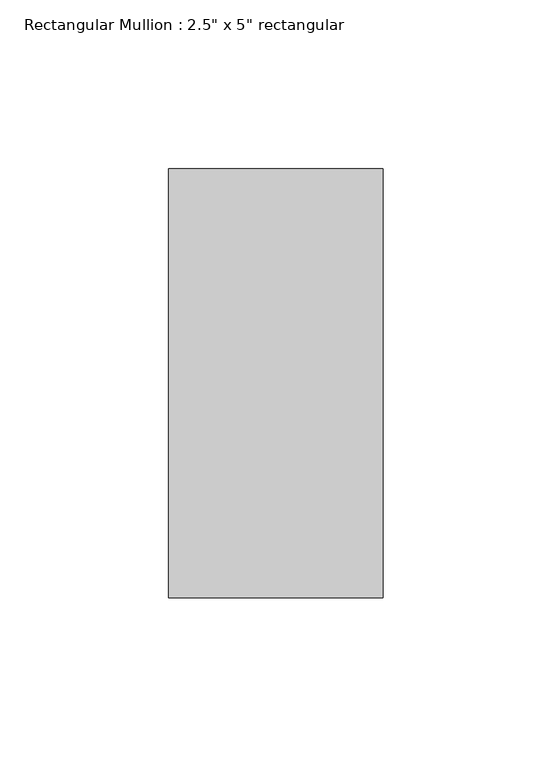
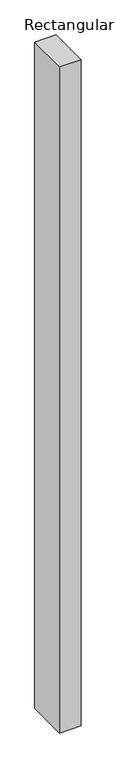
"""IFC4 building model written with IfcOpenShell, lengths in millimetres: member geometry."""

from ifc_helpers import new_model, si_unit, frame, origin, place, context, project, spatial, polyline, outline, extrude, source, transform, mapped, element, save


def member_f51f5eff(model_context):
    return source(origin(), model_context, "Body", "SweptSolid", [
        extrude(outline(polyline([(31.75, 63.5), (31.75, -63.5), (-31.75, -63.5), (-31.75, 63.5), (31.75, 63.5)])), frame((0.0, 0.0, -2080.6846597), z_axis=(0.0, 0.0, 1.0), x_axis=(1.0, 0.0, 0.0)), (0.0, 0.0, 1.0), 2080.6846597),
    ])


if __name__ == "__main__":
    model = new_model("IFC4")
    model_context = context("Model", 3, world=origin())
    ifc_project = project(units=[si_unit("LENGTHUNIT", "METRE", prefix="MILLI")], contexts=[model_context])
    site = spatial("IfcSite", under=ifc_project)
    building = spatial("IfcBuilding", under=site)
    placement = place(None, origin())
    member_shape = member_f51f5eff(model_context)
    element("IfcMember", 1, ObjectType="Rectangular Mullion : 2.5\" x 5\" rectangular", at=placement, inside=building, context=model_context, shape_type="MappedRepresentation", body=[
        mapped(member_shape, transform((0.0, 0.0, 0.0), x_axis=(1.0, 0.0, 0.0), y_axis=(0.0, 1.0, 0.0), z_axis=(0.0, 0.0, 1.0))),
    ])
    save(model, "model.ifc")

# Revit data of these elements
# Type "Rectangular Mullion : 2.5\" x 5\" rectangular"
#   built-in parameter 1007304 = 0.416667 (stored number, unit not read)
#   built-in parameter 1007301 = 0.104167 (stored number, unit not read)
#   built-in parameter 1007300 = 0.104167 (stored number, unit not read)
# Element 1 (IfcMember, "Rectangular Mullion : 2.5\" x 5\" rectangular")
#   Materials on its faces: "Aluminum"
# Materials
#   "Aluminum": class "Metal", colour RGB 247 247 247, transparency 0, Description = "Aluminum 6061", Cost = 0
